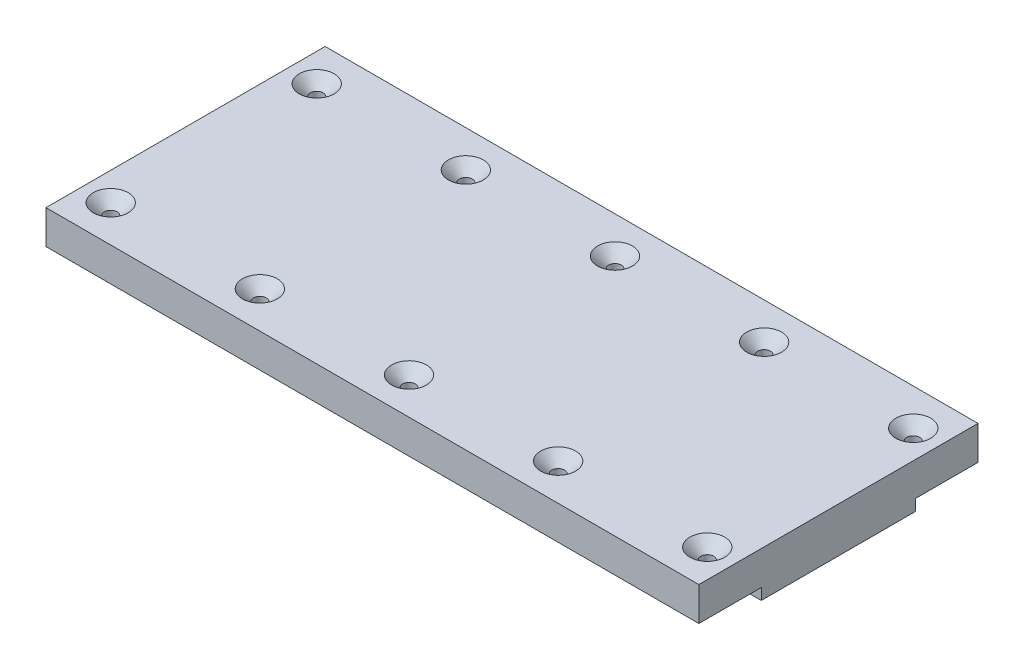
from build123d import *

# Parameters (mm, degrees)
BASE_PLATE_DEPTH           = 580
MOUNTING_HOLES_SKETCH_R    = 5.7
MOUNTING_HOLES_8X_11_DEPTH = 580
HOLE_CHAMFERS_6MM_SIZE     = 9.8


with BuildPart() as part:
    # Plate Profile Sketch → Base Plate (new body)
    with BuildSketch(Plane(origin=(0, 0, 0), x_dir=(0, 0, -1), z_dir=(1, 0, 0))):
        Polygon((-68.5, 0), (68.5, 0), (68.5, 10), (124, 10), (124, 40), (-124, 40), (-124, 10), (-68.5, 10), align=None)
    extrude(amount=BASE_PLATE_DEPTH)

    # Mounting Holes Sketch → Mounting Holes 8xØ11 (cut)
    with BuildSketch(Plane(origin=(0, 40, 0), x_dir=(1, 0, 0), z_dir=(0, 1, 0))):
        with Locations(Location((25, -91.5, 0), (0, 0, 270))):
            Circle(MOUNTING_HOLES_SKETCH_R)
        with Locations(Location((157.5, -91.5, 0), (0, 0, 270))):
            Circle(MOUNTING_HOLES_SKETCH_R)
        with Locations(Location((422.5, -91.5, 0), (0, 0, 270))):
            Circle(MOUNTING_HOLES_SKETCH_R)
        with Locations(Location((555, -91.5, 0), (0, 0, 270))):
            Circle(MOUNTING_HOLES_SKETCH_R)
        with Locations(Location((290, -91.5, 0), (0, 0, 270))):
            Circle(MOUNTING_HOLES_SKETCH_R)
        with Locations(Location((555, 91.5, 0), (0, 0, 270))):
            Circle(MOUNTING_HOLES_SKETCH_R)
        with Locations(Location((422.5, 91.5, 0), (0, 0, 270))):
            Circle(MOUNTING_HOLES_SKETCH_R)
        with Locations(Location((290, 91.5, 0), (0, 0, 270))):
            Circle(MOUNTING_HOLES_SKETCH_R)
        with Locations(Location((157.5, 91.5, 0), (0, 0, 270))):
            Circle(MOUNTING_HOLES_SKETCH_R)
        with Locations(Location((25, 91.5, 0), (0, 0, 270))):
            Circle(MOUNTING_HOLES_SKETCH_R)
    extrude(amount=-MOUNTING_HOLES_8X_11_DEPTH, mode=Mode.SUBTRACT)

    # Hole Chamfers 6mm
    hole_chamfers_6mm_edges = [part.edges().sort_by_distance(p)[0] for p in [
        (25, 40, -97.2),
        (157.5, 40, -97.2),
        (290, 40, -97.2),
        (422.5, 40, -97.2),
        (555, 40, -97.2),
        (157.5, 40, 85.8),
        (422.5, 40, 85.8),
        (555, 40, 85.8),
        (290, 40, 85.8),
        (25, 40, 85.8),
    ]]
    chamfer(hole_chamfers_6mm_edges, length=HOLE_CHAMFERS_6MM_SIZE)


solid = part.part
